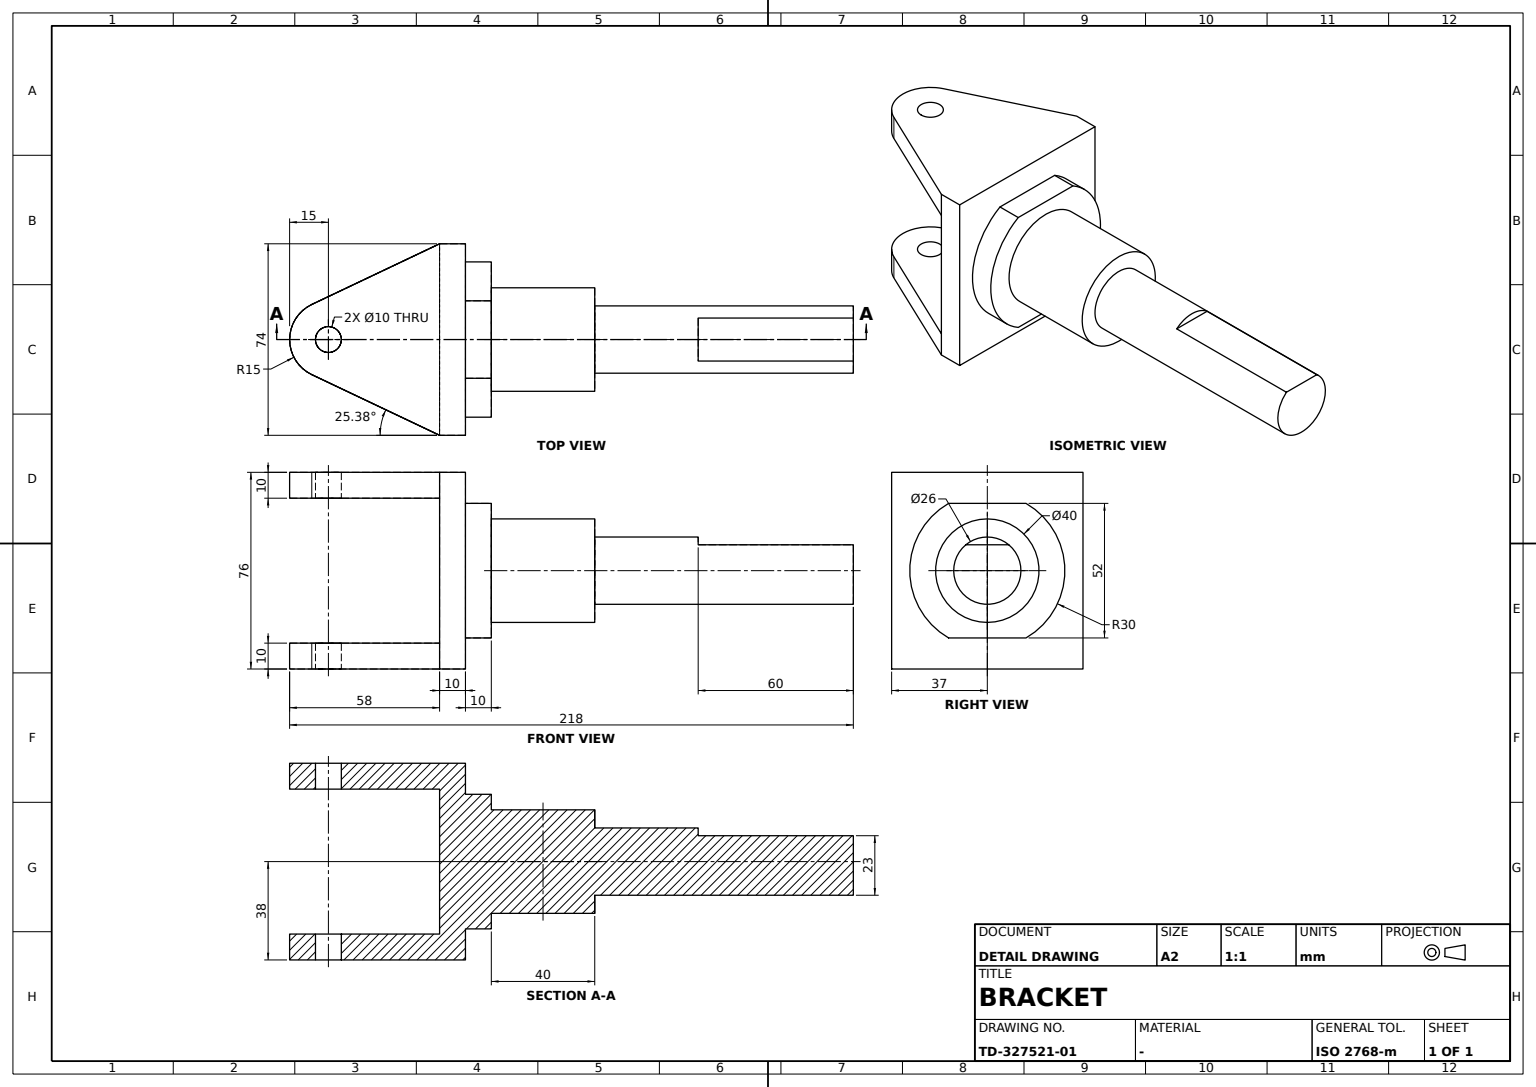
CATIA V5 part; units mm, degrees
sketch "Sketch1" plane through (0, 0, 0) normal (0, 1, 0) x (-1, 0, 0)
  arc A0 (-8.3066, 10) -> (8.3066, 10) centre (0, 0) ccw
  line L0 (8.3066, 10) -> (-8.3066, 10)
  dimension "radius A0" = 13
  constraint horizontal L0 x-axis
extrude "Pad1" add sketch "Sketch1" along normal blind 60
sketch "Sketch2" plane through (0, 0, 0) normal (0, -1, 0) x (1, 0, 0)
  circle A0 centre (0, 0) radius 13
  dimension "radius A0" = 13
extrude "Pad2" add sketch "Sketch2" along normal blind 40
sketch "Sketch3" plane through (0, -40, 0) normal (0, -1, 0) x (1, 0, 0)
  circle A0 centre (0, 0) radius 20
  dimension "radius A0" = 20
extrude "Pad3" add sketch "Sketch3" along normal blind 40
sketch "Sketch4" plane through (0, -80, 0) normal (0, -1, 0) x (1, 0, 0)
  arc A0 (14.9666, -26) -> (14.9666, 26) centre (0, 0) ccw
  line L0 (14.9666, 26) -> (-14.9666, 26)
  point P0 (14.9666, 26)
  point P1 (-14.9666, 26)
  point P2 (-14.9666, -26)
  point P3 (14.9666, -26)
  line L1 (14.9666, -26) -> (-14.9666, -26)
  arc A1 (-14.9666, 26) -> (-14.9666, -26) centre (0, 0) ccw
  dimension "radius A0" = 30
  constraint coincidence P1 A0
  constraint coincidence A0 A1
  constraint horizontal L0 x-axis
  constraint symmetry P1 P2 x-axis
  constraint symmetry P0 P3 x-axis
  constraint symmetry L0 L1 x-axis
extrude "Pad4" add sketch "Sketch4" along normal blind 10
sketch "Sketch5" plane through (0, -90, 0) normal (0, -1, 0) x (1, 0, 0)
  line L0 (37, 38) -> (37, -38)
  line L1 (37, -38) -> (-37, -38)
  line L2 (-37, -38) -> (-37, 38)
  line L3 (-37, 38) -> (37, 38)
  dimension "distance L1 L3" = 76
  dimension "distance L0 L2" = 74
  constraint vertical L0 y-axis
  constraint vertical L2 y-axis
  constraint horizontal L1 x-axis
  constraint horizontal L3 x-axis
  constraint equidistance L0 L2 origin
  constraint equidistance L1 L3 origin
extrude "Pad5" add sketch "Sketch5" along normal blind 10
sketch "Sketch6" plane through (0, 0, 38) normal (0, 0, 1) x (1, 0, 0)
  point P0 (0, -100)
  circle A0 centre (0, -143) radius 5
  arc A1 (-13.5525, -149.4289) -> (13.5525, -149.4289) centre (0, -143) ccw
  line L0 (13.5525, -149.4289) -> (37, -100)
  line L1 (-13.5525, -149.4289) -> (-37, -100)
  line L2 (-37, -100) -> (37, -100)
  dimension "radius A0" = 5
  dimension "radius A1" = 15
  constraint tangency L0 A1
  constraint horizontal L2 x-axis
extrude "Pad6" add sketch "Sketch6" against normal blind 10
sketch "Sketch7" plane through (0, 0, -38) normal (0, 0, -1) x (1, 0, 0)
  point P0 (0, 100)
  circle A0 centre (0, 143) radius 5
  arc A1 (13.5525, 149.4289) -> (-13.5525, 149.4289) centre (0, 143) ccw
  line L0 (-13.5525, 149.4289) -> (-37, 100)
  line L1 (13.5525, 149.4289) -> (37, 100)
  line L2 (-37, 100) -> (37, 100)
  dimension "radius A0" = 5
  dimension "radius A1" = 15
  constraint tangency L0 A1
  constraint tangency L1 A1
  constraint horizontal L2 x-axis
extrude "Pad7" add sketch "Sketch7" against normal blind 10
